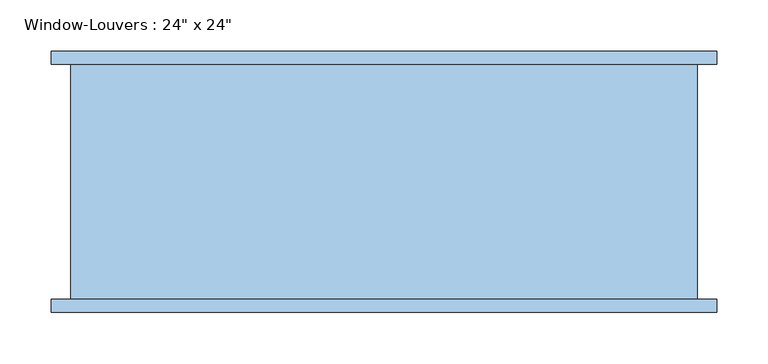
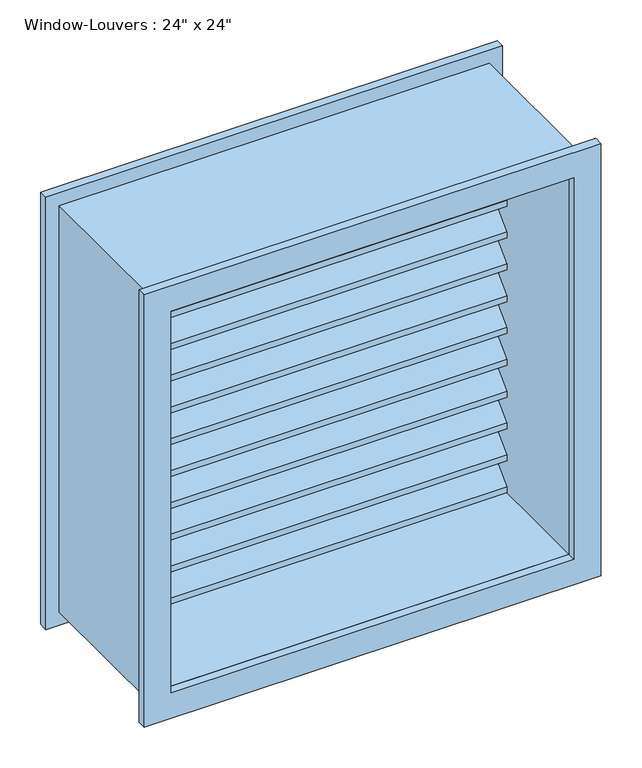
"""IFC4 building model written with IfcOpenShell, lengths in millimetres: window geometry."""

from ifc_helpers import new_model, si_unit, frame, origin, place, context, project, spatial, polyline, outline, extrude, source, transform, mapped, element, save


def window_f2d8fef0(model_context):
    return source(origin(), model_context, "Body", "SweptSolid", [
        extrude(outline(polyline([(107.95, 1419.1754778), (107.95, 1410.1952217), (69.85, 1448.2952217), (31.75, 1410.1952217), (31.75, 1419.1754778), (69.85, 1457.2754778), (107.95, 1419.1754778)])), frame((-285.75, 0.0, 0.0), z_axis=(1.0, 0.0, 0.0), x_axis=(0.0, 1.0, 0.0)), (0.0, 0.0, 1.0), 571.5),
        extrude(outline(polyline([(107.95, 1371.5009557), (107.95, 1362.5206995), (69.85, 1400.6206995), (31.75, 1362.5206995), (31.75, 1371.5009557), (69.85, 1409.6009557), (107.95, 1371.5009557)])), frame((-285.75, 0.0, 0.0), z_axis=(1.0, 0.0, 0.0), x_axis=(0.0, 1.0, 0.0)), (0.0, 0.0, 1.0), 571.5),
        extrude(outline(polyline([(107.95, 1323.8264335), (107.95, 1314.8461774), (69.85, 1352.9461774), (31.75, 1314.8461774), (31.75, 1323.8264335), (69.85, 1361.9264335), (107.95, 1323.8264335)])), frame((-285.75, 0.0, 0.0), z_axis=(1.0, 0.0, 0.0), x_axis=(0.0, 1.0, 0.0)), (0.0, 0.0, 1.0), 571.5),
        extrude(outline(polyline([(107.95, 1276.1519113), (107.95, 1267.1716552), (69.85, 1305.2716552), (31.75, 1267.1716552), (31.75, 1276.1519113), (69.85, 1314.2519113), (107.95, 1276.1519113)])), frame((-285.75, 0.0, 0.0), z_axis=(1.0, 0.0, 0.0), x_axis=(0.0, 1.0, 0.0)), (0.0, 0.0, 1.0), 571.5),
        extrude(outline(polyline([(107.95, 1228.4773891), (107.95, 1219.497133), (69.85, 1257.597133), (31.75, 1219.497133), (31.75, 1228.4773891), (69.85, 1266.5773891), (107.95, 1228.4773891)])), frame((-285.75, 0.0, 0.0), z_axis=(1.0, 0.0, 0.0), x_axis=(0.0, 1.0, 0.0)), (0.0, 0.0, 1.0), 571.5),
        extrude(outline(polyline([(107.95, 1180.802867), (107.95, 1171.8226109), (69.85, 1209.9226109), (31.75, 1171.8226109), (31.75, 1180.802867), (69.85, 1218.902867), (107.95, 1180.802867)])), frame((-285.75, 0.0, 0.0), z_axis=(1.0, 0.0, 0.0), x_axis=(0.0, 1.0, 0.0)), (0.0, 0.0, 1.0), 571.5),
        extrude(outline(polyline([(107.95, 1133.1283448), (107.95, 1124.1480887), (69.85, 1162.2480887), (31.75, 1124.1480887), (31.75, 1133.1283448), (69.85, 1171.2283448), (107.95, 1133.1283448)])), frame((-285.75, 0.0, 0.0), z_axis=(1.0, 0.0, 0.0), x_axis=(0.0, 1.0, 0.0)), (0.0, 0.0, 1.0), 571.5),
        extrude(outline(polyline([(107.95, 1085.4538226), (107.95, 1076.4735665), (69.85, 1114.5735665), (31.75, 1076.4735665), (31.75, 1085.4538226), (69.85, 1123.5538226), (107.95, 1085.4538226)])), frame((-285.75, 0.0, 0.0), z_axis=(1.0, 0.0, 0.0), x_axis=(0.0, 1.0, 0.0)), (0.0, 0.0, 1.0), 571.5),
        extrude(outline(polyline([(107.95, 1037.7793005), (107.95, 1028.7990443), (69.85, 1066.8990443), (31.75, 1028.7990443), (31.75, 1037.7793005), (69.85, 1075.8793005), (107.95, 1037.7793005)])), frame((-285.75, 0.0, 0.0), z_axis=(1.0, 0.0, 0.0), x_axis=(0.0, 1.0, 0.0)), (0.0, 0.0, 1.0), 571.5),
        extrude(outline(polyline([(107.95, 990.1047783), (107.95, 981.1245222), (69.85, 1019.2245222), (31.75, 981.1245222), (31.75, 990.1047783), (69.85, 1028.2047783), (107.95, 990.1047783)])), frame((-285.75, 0.0, 0.0), z_axis=(1.0, 0.0, 0.0), x_axis=(0.0, 1.0, 0.0)), (0.0, 0.0, 1.0), 571.5),
        extrude(outline(polyline([(107.95, 1466.85), (107.95, 1457.8697439), (69.85, 1495.9697439), (31.75, 1457.8697439), (31.75, 1466.85), (69.85, 1504.95), (107.95, 1466.85)])), frame((-285.75, 0.0, 0.0), z_axis=(1.0, 0.0, 0.0), x_axis=(0.0, 1.0, 0.0)), (0.0, 0.0, 1.0), 571.5),
        extrude(outline(polyline([(107.95, 942.4302561), (107.95, 933.45), (69.85, 971.55), (31.75, 933.45), (31.75, 942.4302561), (69.85, 980.5302561), (107.95, 942.4302561)])), frame((-285.75, 0.0, 0.0), z_axis=(1.0, 0.0, 0.0), x_axis=(0.0, 1.0, 0.0)), (0.0, 0.0, 1.0), 571.5),
        extrude(outline(polyline([(1524.0, 304.8), (1524.0, -304.8), (914.4, -304.8), (914.4, 304.8), (1524.0, 304.8)]), holes=[polyline([(1504.95, 285.75), (933.45, 285.75), (933.45, -285.75), (1504.95, -285.75), (1504.95, 285.75)])]), frame((0.0, -120.65, 0.0), z_axis=(0.0, 1.0, 0.0), x_axis=(0.0, 0.0, 1.0)), (0.0, 0.0, 1.0), 228.6),
        extrude(outline(polyline([(1543.05, 323.85), (1543.05, -323.85), (895.35, -323.85), (895.35, 323.85), (1543.05, 323.85)]), holes=[polyline([(1504.95, 285.75), (933.45, 285.75), (933.45, -285.75), (1504.95, -285.75), (1504.95, 285.75)])]), frame((0.0, -133.35, 0.0), z_axis=(0.0, 1.0, 0.0), x_axis=(0.0, 0.0, 1.0)), (0.0, 0.0, 1.0), 12.7),
        extrude(outline(polyline([(1543.05, -323.85), (895.35, -323.85), (895.35, 323.85), (1543.05, 323.85), (1543.05, -323.85)]), holes=[polyline([(1504.95, -285.75), (1504.95, 285.75), (933.45, 285.75), (933.45, -285.75), (1504.95, -285.75)])]), frame((0.0, 107.95, 0.0), z_axis=(0.0, 1.0, 0.0), x_axis=(0.0, 0.0, 1.0)), (0.0, 0.0, 1.0), 12.7),
    ])


if __name__ == "__main__":
    model = new_model("IFC4")
    model_context = context("Model", 3, world=origin())
    ifc_project = project(units=[si_unit("LENGTHUNIT", "METRE", prefix="MILLI")], contexts=[model_context])
    site = spatial("IfcSite", under=ifc_project)
    building = spatial("IfcBuilding", under=site)
    placement = place(None, origin())
    window_shape = window_f2d8fef0(model_context)
    element("IfcWindow", 1, ObjectType="Window-Louvers : 24\" x 24\"", at=placement, inside=building, context=model_context, shape_type="MappedRepresentation", body=[
        mapped(window_shape, transform((0.0, 0.0, 0.0), x_axis=(1.0, 0.0, 0.0), y_axis=(0.0, 1.0, 0.0), z_axis=(0.0, 0.0, 1.0))),
    ])
    save(model, "model.ifc")

# Revit data of these elements
# Type "Window-Louvers : 24\" x 24\""
#   Type Mark = "V1"
#   Construction Type Id = "GSP4R"
#   Assembly Code = "B20"
#   Analytic Construction = "1/8 in Pilkington single glazing"
#   Visual Light Transmittance = 0.9
#   Thermal Resistance (R) = 1.53941 (h·ft²·°F)/BTU
#   Solar Heat Gain Coefficient = 0.78
#   Max Height = 1' - 11.74264"
#   Height = 2' - 0"
#   Heat Transfer Coefficient (U) = 0.6496 BTU/(h·ft²·°F)
#   Blade Width [instance default] = 1' - 10 1/2"
#   Blade Vertical Thickness = 0' - 0.35355"
#   Blade Thickness = 0' - 0 1/4"
#   Blade Spacing = 0' - 1 1/2"
#   Blade Height = 0' - 1.85355"
#   Blade Depth = 0' - 3"
#   Blade Angle = 45.00°
#   Default Sill Height = 3' - 0"
#   Trim Projection_Exterior = 0' - 0 1/2"
#   Trim Projection_Interior = 0' - 0 1/2"
#   Trim Width_Exterior = 0' - 1 1/2"
#   Trim Width_Interior = 0' - 1 1/2"
#   Width = 2' - 0"
#   Max Blade Count = 12
#   Define Thermal Properties by = 1
#   Blade Count = 12
#   Frame Material = Birch
#   Louver Material = Birch
#   Trim Exterior Material = Birch
#   Trim Interior Material = Birch
#   Wall Closure = (empty or 0)
# Element 1 (IfcWindow, "Window-Louvers : 24\" x 24\"")
#   Materials on its faces: "Birch"
# Materials
#   "Birch": class "Wood", colour RGB 224 178 126, transparency 0, Description = "Betula Alleghaniensis", Cost = 0
